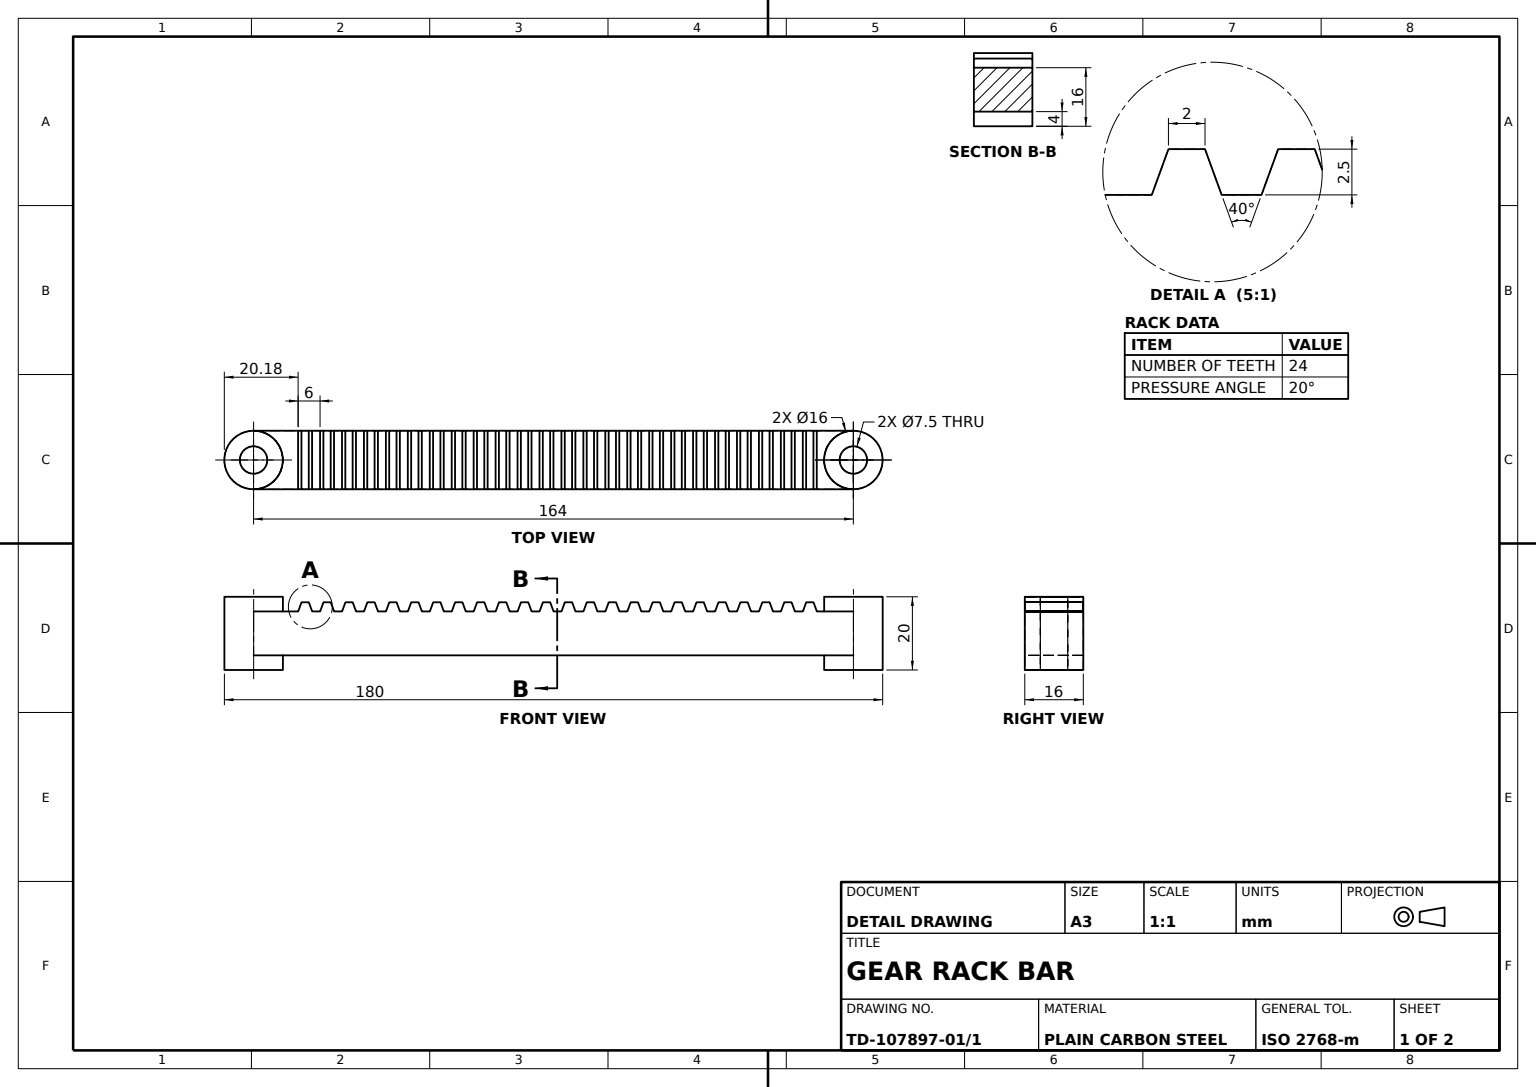
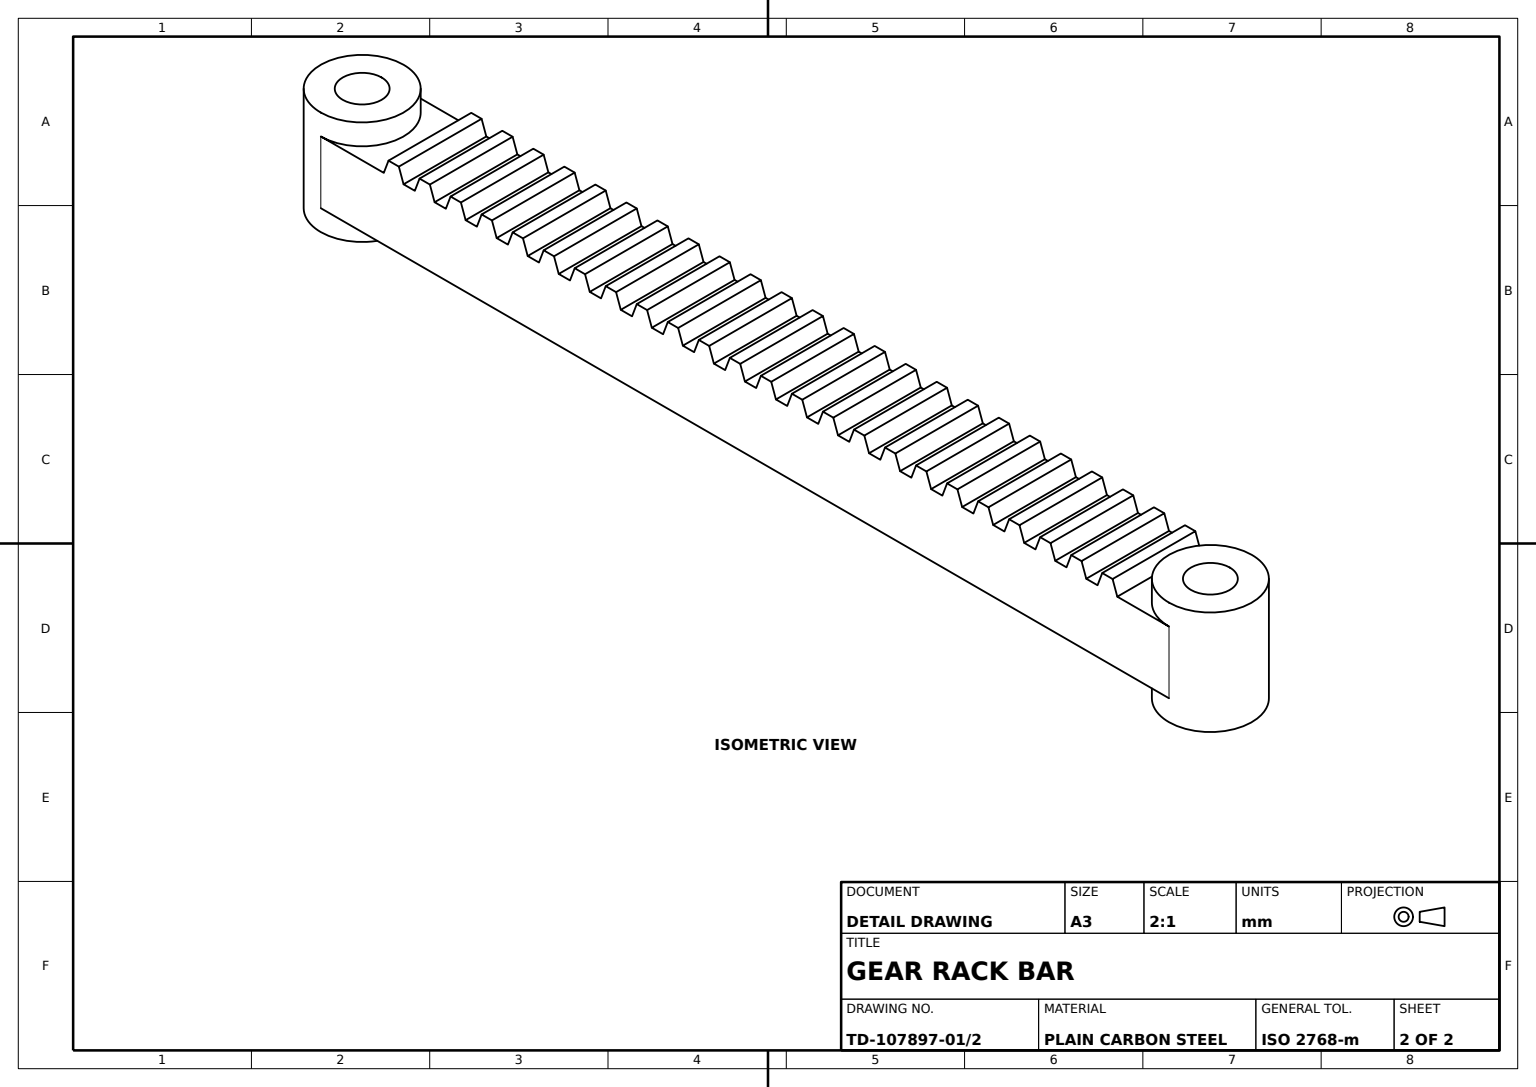
from build123d import *

# Parameters (mm, degrees)
END_BOSSES_SKETCH_R   = 8
END_BOSSES_SKETCH_R_2 = 3.75
END_BOSSES_DEPTH      = 20
END_BOSSES_2_DEPTH    = 20
RACK_TEETH_24X_DEPTH  = 8
PIN_START             = -36
PIN_HOLES_SKETCH_R    = 3.75
PIN_HOLES_2X_DEPTH    = 36


with BuildPart() as part:
    # End Bosses Sketch → End Bosses (new body)
    with BuildSketch(Plane(origin=(0, 0, 0), x_dir=(1, 0, 0), z_dir=(0, 1, 0))):
        with Locations(Location((-82, 0, 0), (0, 0, 270))):
            Circle(END_BOSSES_SKETCH_R)
        with Locations(Location((-82, 0, 0), (0, 0, 270))):
            Circle(END_BOSSES_SKETCH_R_2, mode=Mode.SUBTRACT)
    extrude(amount=END_BOSSES_DEPTH)



with BuildPart() as body_2:
    # End Bosses Sketch → End Bosses 2 (new body)
    with BuildSketch(Plane(origin=(0, 0, 0), x_dir=(1, 0, 0), z_dir=(0, 1, 0))):
        with Locations(Location((82, 0, 0), (0, 0, 270))):
            Circle(END_BOSSES_SKETCH_R)
        with Locations(Location((82, 0, 0), (0, 0, 270))):
            Circle(END_BOSSES_SKETCH_R_2, mode=Mode.SUBTRACT)
    extrude(amount=END_BOSSES_2_DEPTH)


with BuildPart() as part_1:
    add(part.part)

    add(body_2.part)  # Rack Teeth 24x merges body 2
    # Rack Tooth Profile Sketch → Rack Teeth 24x (add, symmetric)
    with BuildSketch(Plane.XY):
        Polygon((-82, 4), (82, 4), (82, 16), (72, 16), (71.090074414, 18.5), (69.090074414, 18.5), (68.180148829, 16), (66, 16), (65.090074414, 18.5), (63.090074414, 18.5), (62.180148829, 16), (60, 16), (59.090074414, 18.5), (57.090074414, 18.5), (56.180148829, 16), (54, 16), (53.090074414, 18.5), (51.090074414, 18.5), (50.180148829, 16), (48, 16), (47.090074414, 18.5), (45.090074414, 18.5), (44.180148829, 16), (42, 16), (41.090074414, 18.5), (39.090074414, 18.5), (38.180148829, 16), (36, 16), (35.090074414, 18.5), (33.090074414, 18.5), (32.180148829, 16), (30, 16), (29.090074414, 18.5), (27.090074414, 18.5), (26.180148829, 16), (24, 16), (23.090074414, 18.5), (21.090074414, 18.5), (20.180148829, 16), (18, 16), (17.090074414, 18.5), (15.090074414, 18.5), (14.180148829, 16), (12, 16), (11.090074414, 18.5), (9.090074414, 18.5), (8.180148829, 16), (6, 16), (5.090074414, 18.5), (3.090074414, 18.5), (2.180148829, 16), (0, 16), (-0.909925586, 18.5), (-2.909925586, 18.5), (-3.819851171, 16), (-6, 16), (-6.909925586, 18.5), (-8.909925586, 18.5), (-9.819851171, 16), (-12, 16), (-12.909925586, 18.5), (-14.909925586, 18.5), (-15.819851171, 16), (-18, 16), (-18.909925586, 18.5), (-20.909925586, 18.5), (-21.819851171, 16), (-24, 16), (-24.909925586, 18.5), (-26.909925586, 18.5), (-27.819851171, 16), (-30, 16), (-30.909925586, 18.5), (-32.909925586, 18.5), (-33.819851171, 16), (-36, 16), (-36.909925586, 18.5), (-38.909925586, 18.5), (-39.819851171, 16), (-42, 16), (-42.909925586, 18.5), (-44.909925586, 18.5), (-45.819851171, 16), (-48, 16), (-48.909925586, 18.5), (-50.909925586, 18.5), (-51.819851171, 16), (-54, 16), (-54.909925586, 18.5), (-56.909925586, 18.5), (-57.819851171, 16), (-60, 16), (-60.909925586, 18.5), (-62.909925586, 18.5), (-63.819851171, 16), (-66, 16), (-66.909925586, 18.5), (-68.909925586, 18.5), (-69.819851171, 16), (-82, 16), align=None)
    extrude(amount=RACK_TEETH_24X_DEPTH, both=True)

    # Pin Holes Sketch → Pin Holes 2x (cut)
    with BuildSketch(Plane(origin=(0, 20, 0), x_dir=(1, 0, 0), z_dir=(0, 1, 0)).offset(PIN_START)):
        with Locations(Location((-82, 0, 0), (0, 0, 270))):
            Circle(PIN_HOLES_SKETCH_R)
        with Locations(Location((82, 0, 0), (0, 0, 270))):
            Circle(PIN_HOLES_SKETCH_R)
    extrude(amount=PIN_HOLES_2X_DEPTH, mode=Mode.SUBTRACT)


solid = part_1.part
